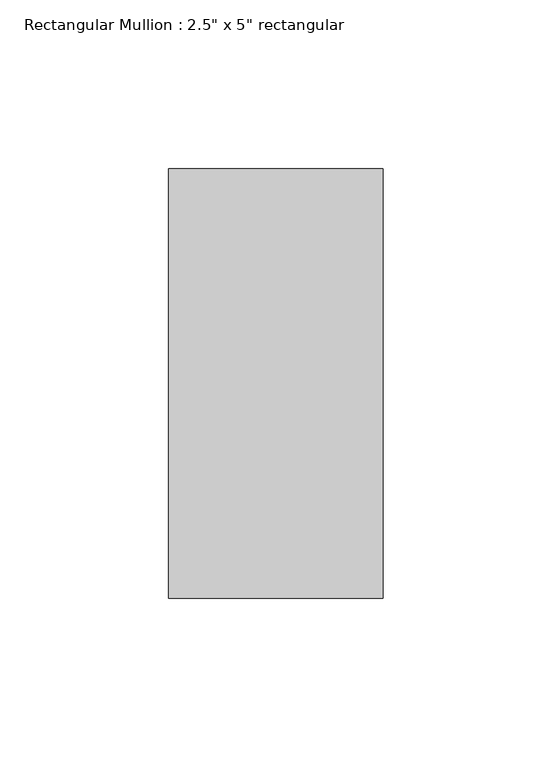
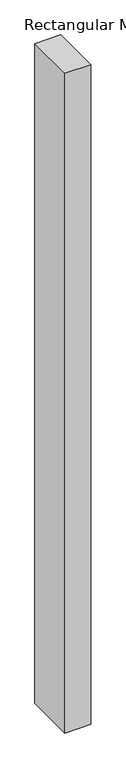
"""IFC4 building model written with IfcOpenShell, lengths in millimetres: member geometry."""

from ifc_helpers import new_model, si_unit, frame, origin, place, context, project, spatial, polyline, outline, extrude, source, transform, mapped, element, save


def member_7bc42366(model_context):
    return source(origin(), model_context, "Body", "SweptSolid", [
        extrude(outline(polyline([(0.0, 63.5), (0.0, -63.5), (-63.5, -63.5), (-63.5, 63.5), (0.0, 63.5)])), frame((0.0, 0.0, -1701.8), z_axis=(0.0, 0.0, 1.0), x_axis=(1.0, 0.0, 0.0)), (0.0, 0.0, 1.0), 1701.8),
    ])


if __name__ == "__main__":
    model = new_model("IFC4")
    model_context = context("Model", 3, world=origin())
    ifc_project = project(units=[si_unit("LENGTHUNIT", "METRE", prefix="MILLI")], contexts=[model_context])
    site = spatial("IfcSite", under=ifc_project)
    building = spatial("IfcBuilding", under=site)
    placement = place(None, origin())
    member_shape = member_7bc42366(model_context)
    element("IfcMember", 1, ObjectType="Rectangular Mullion : 2.5\" x 5\" rectangular", at=placement, inside=building, context=model_context, shape_type="MappedRepresentation", body=[
        mapped(member_shape, transform((0.0, 0.0, 0.0), x_axis=(1.0, 0.0, 0.0), y_axis=(0.0, 1.0, 0.0), z_axis=(0.0, 0.0, 1.0))),
    ])
    save(model, "model.ifc")

# Revit data of these elements
# Type "Rectangular Mullion : 2.5\" x 5\" rectangular"
#   built-in parameter 1007304 = 0.416667 (stored number, unit not read)
#   built-in parameter 1007301 = 0.104167 (stored number, unit not read)
#   built-in parameter 1007300 = 0.104167 (stored number, unit not read)
# Element 1 (IfcMember, "Rectangular Mullion : 2.5\" x 5\" rectangular")
#   Materials on its faces: "Aluminum"
# Materials
#   "Aluminum": class "Metal", colour RGB 247 247 247, transparency 0, Description = "Aluminum 6061", Cost = 0
